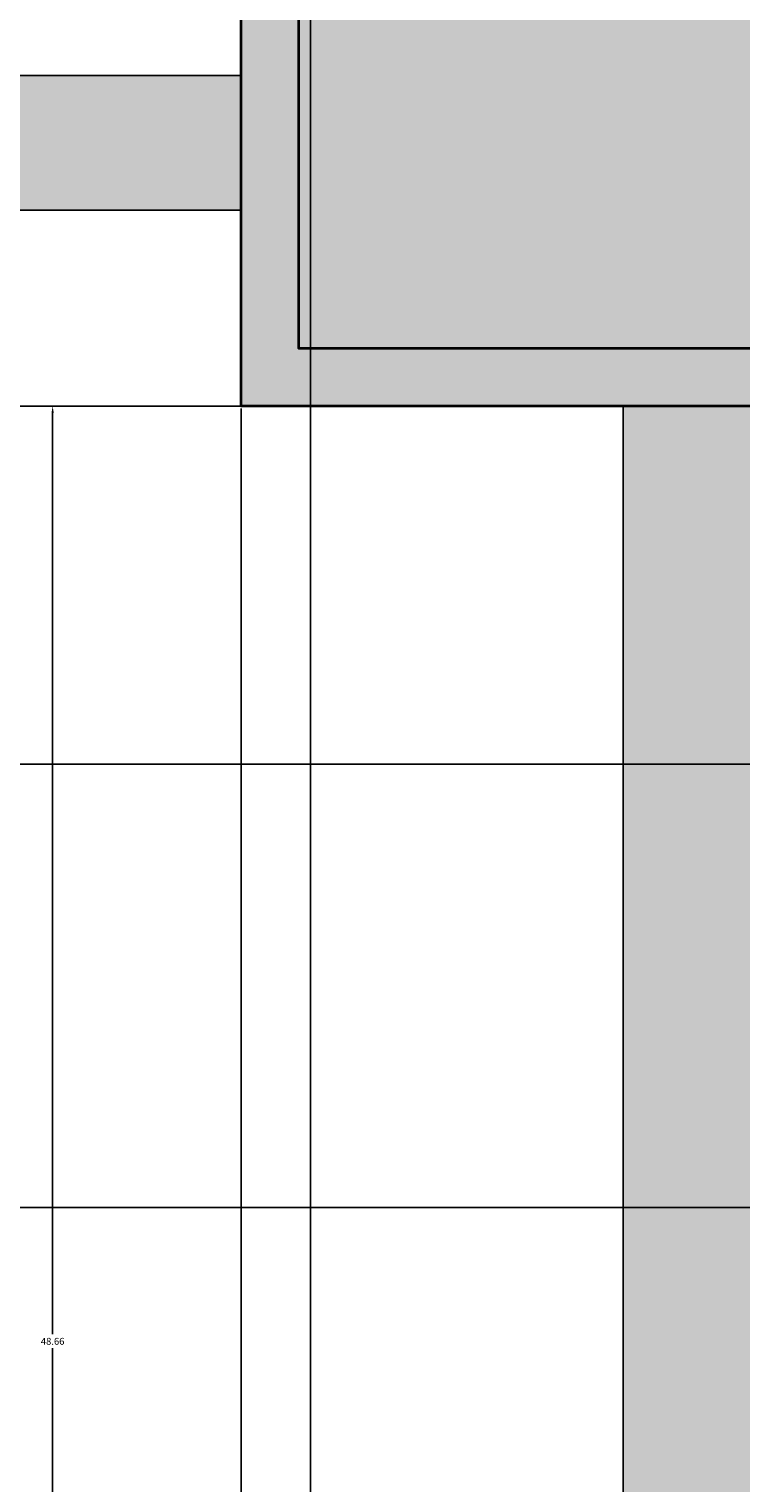
# Model space of a CAD drawing. Units: millimetres. Extents: x -11 to 280, y -4 to 208.
# Tile 11 of 55: x 24 to 42, y 126 to 164. Entities that reach past the tile are written whole.
import ezdxf

# ---------------------------------------------------------------- set-up
doc = ezdxf.new("R2010")
doc.units = ezdxf.units.MM
for name, color, linetype, lineweight in [('M-DIMS', 2, 'Continuous', 18), ('M-HYDR-EQPM', 7, 'Continuous', 35), ('M-HYDR-EQPM-PATT', 252, 'Continuous', 13), ('M-HYDR-RETN', 7, 'Continuous', 25), ('M-HYDR-SUCT', 7, 'Continuous', 25)]:
    doc.layers.add(name, color=color, linetype=linetype, lineweight=lineweight)
doc.layers.add('M-HYDR-RETN-PATT', color=114, linetype='Continuous', lineweight=13, true_color=0x139b48)
doc.layers.add('M-HYDR-SUCT-PATT', color=221, linetype='Continuous', lineweight=13, true_color=0xff7fdf)
doc.styles.get("Standard").update_dxf_attribs({"font": 'arial.ttf'})
doc.dimstyles.get("Standard").update_dxf_attribs({"dimtxt": 0.18, "dimasz": 0.18, "dimexe": 0.18, "dimexo": 0.0625, "dimgap": 0.09, "dimtad": 0, "dimtih": 1, "dimtoh": 1, "dimdec": 4, "dimzin": 0, "dimdsep": 46, "dimtxsty": 'Standard', "dimcen": 0.09, "dimadec": 0, "dimazin": 0, "dimtfac": 1, "dimtdec": 4, "dimtofl": 0, "dimtmove": 0, "dimatfit": 3, "dimfxl": 1, "dimtolj": 1, "dimtzin": 0, "dimarcsym": 0})

# ---------------------------------------------------------------- blocks, each defined once
blk = doc.blocks.new('*D5')
at = {"layer": 'Defpoints', "color": 0, "transparency": 16777216}
for p in [(24.759, 192.645), (-10.087, 11.435), (261.686, 11.435)]:
    blk.add_point(p, dxfattribs=at)
at = {"layer": 'M-DIMS', "color": 0, "lineweight": -2, "transparency": 16777216}
for p, q in [((24.696, 192.645), (-10.267, 192.645)), ((-10.087, 192.465), (-10.087, 102.222)), ((-10.087, 11.615), (-10.087, 101.858)), ((261.624, 11.435), (-10.267, 11.435))]:
    blk.add_line(p, q, dxfattribs=at)
at = {"layer": 'M-DIMS', "color": 0, "transparency": 16777216}
for points in [[(-10.117, 192.465), (-10.057, 192.465), (-10.087, 192.645)], [(-10.117, 11.615), (-10.057, 11.615), (-10.087, 11.435)]]:
    blk.add_solid(points, dxfattribs=at)
at = {"layer": 'M-DIMS', "color": 0, "transparency": 16777216, "insert": (-10.087, 102.04), "char_height": 0.18, "attachment_point": 5}
blk.add_mtext('\\A1;181.2', dxfattribs=at)
blk = doc.blocks.new('*D8')
at = {"layer": 'Defpoints', "color": 0, "transparency": 16777216}
for p in [(29.201, 177.431), (14.47, 162.581), (29.201, 162.581)]:
    blk.add_point(p, dxfattribs=at)
at = {"layer": 'M-DIMS', "color": 0, "lineweight": -2, "transparency": 16777216}
for p, q in [((14.47, 162.644), (14.47, 177.611)), ((14.65, 177.431), (21.451, 177.431)), ((29.021, 177.431), (22.221, 177.431)), ((29.201, 162.644), (29.201, 177.611))]:
    blk.add_line(p, q, dxfattribs=at)
at = {"layer": 'M-DIMS', "color": 0, "transparency": 16777216}
for points in [[(14.65, 177.461), (14.65, 177.401), (14.47, 177.431)], [(29.021, 177.461), (29.021, 177.401), (29.201, 177.431)]]:
    blk.add_solid(points, dxfattribs=at)
at = {"layer": 'M-DIMS', "color": 0, "transparency": 16777216, "insert": (21.836, 177.431), "char_height": 0.18, "attachment_point": 5}
blk.add_mtext('\\A1;14.73', dxfattribs=at)
blk = doc.blocks.new('*D9')
at = {"layer": 'Defpoints', "color": 0, "transparency": 16777216}
for p in [(78.827, 207.495), (31.006, 98.021), (78.827, 98.149)]:
    blk.add_point(p, dxfattribs=at)
at = {"layer": 'M-DIMS', "color": 0, "lineweight": -2, "transparency": 16777216}
for p, q in [((31.006, 98.084), (31.006, 207.675)), ((31.186, 207.495), (54.52, 207.495)), ((78.647, 207.495), (55.313, 207.495)), ((78.827, 98.212), (78.827, 207.675))]:
    blk.add_line(p, q, dxfattribs=at)
at = {"layer": 'M-DIMS', "color": 0, "transparency": 16777216}
for points in [[(31.186, 207.525), (31.186, 207.465), (31.006, 207.495)], [(78.647, 207.525), (78.647, 207.465), (78.827, 207.495)]]:
    blk.add_solid(points, dxfattribs=at)
at = {"layer": 'M-DIMS', "color": 0, "transparency": 16777216, "insert": (54.917, 207.495), "char_height": 0.18, "attachment_point": 5}
blk.add_mtext('\\A1;47.82', dxfattribs=at)
blk = doc.blocks.new('*D10')
at = {"layer": 'Defpoints', "color": 0, "transparency": 16777216}
for p in [(24.295, 153.977), (39.145, 153.977), (39.145, 105.314)]:
    blk.add_point(p, dxfattribs=at)
at = {"layer": 'M-DIMS', "color": 0, "lineweight": -2, "transparency": 16777216}
for p, q in [((39.083, 153.977), (24.115, 153.977)), ((24.295, 153.797), (24.295, 129.827)), ((24.295, 105.494), (24.295, 129.464)), ((39.083, 105.314), (24.115, 105.314))]:
    blk.add_line(p, q, dxfattribs=at)
at = {"layer": 'M-DIMS', "color": 0, "transparency": 16777216}
for points in [[(24.265, 153.797), (24.325, 153.797), (24.295, 153.977)], [(24.265, 105.494), (24.325, 105.494), (24.295, 105.314)]]:
    blk.add_solid(points, dxfattribs=at)
at = {"layer": 'M-DIMS', "color": 0, "transparency": 16777216, "insert": (24.295, 129.645), "char_height": 0.18, "attachment_point": 5}
blk.add_mtext('\\A1;48.66', dxfattribs=at)
blk = doc.blocks.new('*D14')
at = {"layer": 'Defpoints', "color": 0, "transparency": 16777216}
for p in [(-10.087, 144.661), (205.531, 144.661), (226.511, 133.123)]:
    blk.add_point(p, dxfattribs=at)
at = {"layer": 'M-DIMS', "color": 0, "lineweight": -2, "transparency": 16777216}
for p, q in [((205.469, 144.661), (-10.267, 144.661)), ((-10.087, 144.481), (-10.087, 139.074)), ((-10.087, 133.303), (-10.087, 138.71)), ((226.448, 133.123), (-10.267, 133.123))]:
    blk.add_line(p, q, dxfattribs=at)
at = {"layer": 'M-DIMS', "color": 0, "transparency": 16777216}
for points in [[(-10.117, 144.481), (-10.057, 144.481), (-10.087, 144.661)], [(-10.117, 133.303), (-10.057, 133.303), (-10.087, 133.123)]]:
    blk.add_solid(points, dxfattribs=at)
at = {"layer": 'M-DIMS', "color": 0, "transparency": 16777216, "insert": (-10.087, 138.892), "char_height": 0.18, "attachment_point": 5}
blk.add_mtext('\\A1;11.538', dxfattribs=at)
blk = doc.blocks.new('*D23')
at = {"layer": 'Defpoints', "color": 0, "transparency": 16777216}
for p in [(29.201, 153.977), (66.388, 153.977), (66.388, -3.415)]:
    blk.add_point(p, dxfattribs=at)
at = {"layer": 'M-DIMS', "color": 0, "lineweight": -2, "transparency": 16777216}
for p, q in [((29.201, 153.914), (29.201, -3.595)), ((66.388, 153.914), (66.388, -3.595)), ((29.381, -3.415), (47.331, -3.415)), ((66.208, -3.415), (48.258, -3.415))]:
    blk.add_line(p, q, dxfattribs=at)
at = {"layer": 'M-DIMS', "color": 0, "transparency": 16777216}
for points in [[(29.381, -3.385), (29.381, -3.445), (29.201, -3.415)], [(66.208, -3.385), (66.208, -3.445), (66.388, -3.415)]]:
    blk.add_solid(points, dxfattribs=at)
at = {"layer": 'M-DIMS', "color": 0, "transparency": 16777216, "insert": (47.795, -3.415), "char_height": 0.18, "attachment_point": 5}
blk.add_mtext('\\A1;37.186', dxfattribs=at)
blk = doc.blocks.new('*D24')
at = {"layer": 'Defpoints', "color": 0, "transparency": 16777216}
for p in [(14.351, 179.241), (29.201, 179.241), (29.201, 153.977)]:
    blk.add_point(p, dxfattribs=at)
at = {"layer": 'M-DIMS', "color": 0, "lineweight": -2, "transparency": 16777216}
for p, q in [((29.139, 179.241), (14.171, 179.241)), ((14.351, 179.061), (14.351, 166.791)), ((14.351, 154.157), (14.351, 166.427)), ((29.139, 153.977), (14.171, 153.977))]:
    blk.add_line(p, q, dxfattribs=at)
at = {"layer": 'M-DIMS', "color": 0, "transparency": 16777216}
for points in [[(14.321, 179.061), (14.381, 179.061), (14.351, 179.241)], [(14.321, 154.157), (14.381, 154.157), (14.351, 153.977)]]:
    blk.add_solid(points, dxfattribs=at)
at = {"layer": 'M-DIMS', "color": 0, "transparency": 16777216, "insert": (14.351, 166.609), "char_height": 0.18, "attachment_point": 5}
blk.add_mtext('\\A1;25.264', dxfattribs=at)

msp = doc.modelspace()

# ---------------------------------------------------------------- hatches: boundary and pattern name
at = {"layer": 'M-HYDR-EQPM-PATT'}
h = msp.add_hatch(color=256, dxfattribs=at)
h.set_gradient(color1=(153, 153, 0), color2=(255, 255, 0), tint=1, name='INVCYLINDER')
h.paths.add_polyline_path([(64.8875, 177.7412), (30.7015, 177.7412), (30.7015, 155.4768), (64.8875, 155.4768)])
h.paths.add_polyline_path([(52.0736, 184.1929), (52.0736, 192.645), (24.7588, 192.645), (24.7588, 184.1929), (34.0713, 184.1929), (34.0713, 179.2412), (35.5061, 179.2412), (35.5061, 185.6276), (26.1935, 185.6276), (26.1935, 191.2103), (50.6389, 191.2103), (50.6389, 185.6276), (41.792, 185.6276), (41.792, 179.2412), (43.2268, 179.2412), (43.2268, 184.1929)])
h = msp.add_hatch(color=256, dxfattribs=at)
h.set_gradient(color1=(153, 153, 0), color2=(153, 153, 0), tint=1, name='INVCYLINDER')
h.paths.add_polyline_path([(26.1935, 191.2103), (26.1935, 185.6276), (35.5061, 185.6276), (35.5061, 179.2412), (41.792, 179.2412), (41.792, 185.6276), (50.6389, 185.6276), (50.6389, 191.2103)])
h.paths.add_polyline_path([(29.2015, 153.9768), (66.3875, 153.9768), (66.3875, 179.2412), (29.2015, 179.2412)])
h.paths.add_polyline_path([(30.7015, 177.7412), (64.8875, 177.7412), (64.8875, 155.4768), (30.7015, 155.4768)], flags=16)
at = {"layer": 'M-HYDR-RETN-PATT'}
h = msp.add_hatch(color=256, dxfattribs=at)
h.set_gradient(color1=(19, 155, 72), color2=(19, 155, 72), tint=1)
h.paths.add_polyline_path([(17.9701, 159.0814), (29.2015, 159.0814), (29.2015, 162.5814), (14.4701, 162.5814), (14.4701, 98.0213), (17.9701, 98.0213)])
h.paths.add_polyline_path([(17.9701, 84.4261), (14.4701, 84.4261), (14.4701, 54.3099), (156.2446, 54.3099), (156.2446, 57.8099), (17.9701, 57.8099)])
h.paths.add_polyline_path([(120.5137, 74.3991), (17.9701, 74.3991), (17.9701, 70.8991), (120.5137, 70.8991)], flags=17)
h.paths.add_polyline_path([(184.7092, 75.04, 0.4142136), (179.7092, 80.04), (156.2446, 80.04), (156.2446, 57.8099), (156.2446, 54.3099), (156.2446, 43.5991), (159.7446, 43.5991), (159.7446, 57.8099), (159.7446, 76.54), (176.2092, 76.54, -0.4142136), (181.2092, 71.54), (181.2092, 57.8099), (159.7446, 57.8099), (159.7446, 54.3099), (184.7092, 54.3099)])
at = {"layer": 'M-HYDR-SUCT-PATT'}
h = msp.add_hatch(color=256, dxfattribs=at)
h.set_gradient(color1=(255, 127, 223), color2=(255, 127, 223), tint=1, name='INVCYLINDER')
h.paths.add_polyline_path([(91.3629, 155.4768), (91.3629, 132.4768), (58.3629, 132.4768), (58.3629, 153.9768), (54.8629, 153.9768), (54.8629, 128.9768), (94.8629, 128.9768), (94.8629, 151.9768), (205.5315, 151.9768), (205.5315, 155.4768)])
h.paths.add_polyline_path([(91.3, 114.9452, 1), (78.8273, 114.9452), (78.8273, 108.8141), (42.6453, 108.8141), (42.6453, 153.9768), (39.1453, 153.9768), (39.1453, 105.3141), (78.8273, 105.3141), (78.8273, 98.1491, 1), (91.3, 98.1491), (91.3, 105.3141), (95.5776, 105.3141), (95.5776, 108.8141), (91.3, 108.8141)])
h.paths.add_polyline_path([(228.7, 138.4081), (232.2, 138.4081), (232.2, 144.6609), (228.7, 144.6609)])
h.paths.add_polyline_path([(253.1005, 151.9768, 1), (253.1005, 155.4768), (252.6001, 155.4768), (253.5249, 153.991, -0.1401047), (253.6005, 153.7268, -0.7542249), (252.676, 153.4626), (251.4221, 155.4768), (236.9353, 155.4768), (236.9353, 151.9768)])
h.paths.add_polyline_path([(30.8182, 40.7626), (30.8182, 36.7626), (60.8182, 36.7626), (60.8182, 40.7626)])

# ---------------------------------------------------------------- linework, layer by layer
at = {"layer": 'M-HYDR-EQPM'}
for points in [[(29.2015, 179.2412), (66.3875, 179.2412), (66.3875, 153.9768), (29.2015, 153.9768)], [(30.7015, 177.7412), (64.8875, 177.7412), (64.8875, 155.4768), (30.7015, 155.4768)]]:
    msp.add_lwpolyline(points, close=True, dxfattribs=at)
at = {"layer": 'M-HYDR-RETN'}
for p, q in [((29.2015, 162.5814), (14.4701, 162.5814)), ((29.2015, 159.0814), (17.9701, 159.0814))]:
    msp.add_line(p, q, dxfattribs=at)
at = {"layer": 'M-HYDR-SUCT'}
msp.add_lwpolyline([(78.8273, 105.3141), (39.1453, 105.3141), (39.1453, 153.9768)], dxfattribs=at)

# ---------------------------------------------------------------- dimensions: what is measured, and where the dimension line sits
at = {"layer": 'M-DIMS'}
for base, p1, p2, override, picture, middle in [((78.8273, 207.495), (31.0059, 98.0213), (78.8273, 98.1491), {"dimdec": 2, "dimlfac": 1, "dimrnd": 0, "dimzin": 0, "dimdsep": 46, "dimlunit": 2}, '*D9', (54.9166, 207.495)), ((29.2015, 177.4314), (14.4701, 162.5814), (29.2015, 162.5814), {"dimdec": 2, "dimlfac": 1, "dimrnd": 0, "dimzin": 0, "dimdsep": 46, "dimlunit": 2}, '*D8', (21.8358, 177.4314)), ((66.3875, -3.4154), (29.2015, 153.9768), (66.3875, 153.9768), {"dimdec": 3, "dimlfac": 1, "dimrnd": 0, "dimzin": 0, "dimdsep": 46, "dimlunit": 2}, '*D23', (47.7945, -3.4154))]:
    dim = msp.add_linear_dim(base=base, p1=p1, p2=p2, dimstyle='Standard', override=override, dxfattribs=at)
    dim.commit()
    dim.dimension.update_dxf_attribs({"geometry": picture, "text_midpoint": middle})
for base, p1, p2, override, picture, middle in [((-10.0865, 11.4346), (24.7588, 192.645), (261.6863, 11.4346), {"dimdec": 1, "dimlfac": 1, "dimrnd": 0, "dimzin": 0, "dimdsep": 46, "dimlunit": 2}, '*D5', (-10.0865, 102.0398)), ((14.3515, 179.2412), (29.2015, 153.9768), (29.2015, 179.2412), {"dimdec": 3, "dimlfac": 1, "dimrnd": 0, "dimzin": 0, "dimdsep": 46, "dimlunit": 2}, '*D24', (14.3515, 166.609)), ((24.2953, 153.9768), (39.1453, 105.3141), (39.1453, 153.9768), {"dimdec": 2, "dimlfac": 1, "dimrnd": 0, "dimzin": 0, "dimdsep": 46, "dimlunit": 2}, '*D10', (24.2953, 129.6454)), ((-10.0865, 144.6609), (226.5106, 133.1228), (205.5315, 144.6609), {"dimdec": 3, "dimlfac": 1, "dimrnd": 0, "dimzin": 0, "dimdsep": 46, "dimlunit": 2}, '*D14', (-10.0865, 138.8918))]:
    dim = msp.add_linear_dim(base=base, p1=p1, p2=p2, angle=90, dimstyle='Standard', override=override, dxfattribs=at)
    dim.commit()
    dim.dimension.update_dxf_attribs({"geometry": picture, "text_midpoint": middle})

doc.saveas('drawing.dxf')
